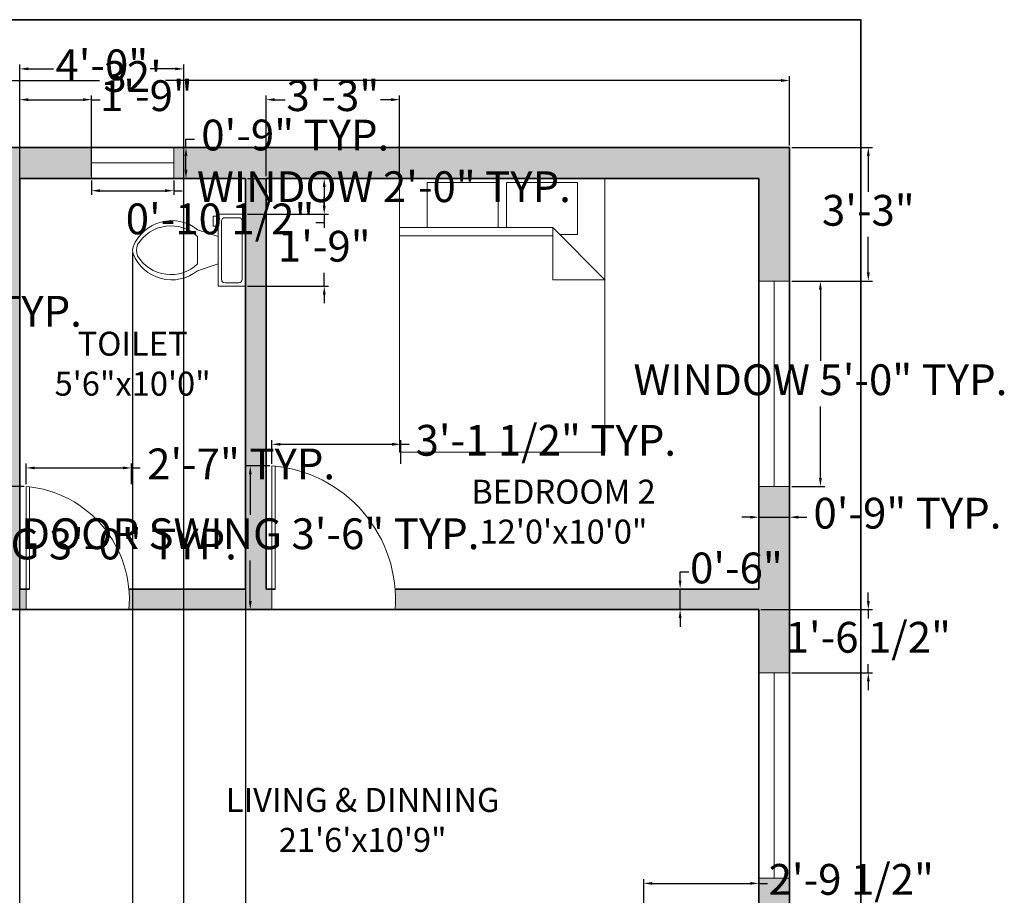
# Model space of a CAD drawing. Units: inches. Extents: x 1649 to 2193, y 1782 to 2280.
# Tile 3 of 3: x 1905 to 2193, y 2024 to 2280. Entities that reach past the tile are written whole.
import ezdxf

# ---------------------------------------------------------------- set-up
doc = ezdxf.new("R2010")
doc.units = ezdxf.units.IN
for name, color, linetype, lineweight in [('A-ANNO-DIMS', 2, 'Continuous', 18), ('A-ANNO-TTLB', 7, 'Continuous', 35), ('A-AREA-IDEN', 7, 'Continuous', 25), ('A-DOOR', 3, 'Continuous', 18), ('A-FLOR-FIXT', 9, 'Continuous', 18), ('A-FURN', 8, 'Continuous', 18), ('A-GLAZ', 4, 'Continuous', 18), ('A-WALL', 7, 'Continuous', 35)]:
    doc.layers.add(name, color=color, linetype=linetype, lineweight=lineweight)
doc.layers.add('A-WALL-PATT', color=18, linetype='Continuous', lineweight=13, true_color=0x000000)
doc.styles.get("Standard").update_dxf_attribs({"font": 'arial.ttf'})
doc.dimstyles.new('ISO-25', dxfattribs={"dimtxt": 9, "dimasz": 2.5, "dimexe": 1.25, "dimexo": 0.625, "dimgap": 2, "dimtad": 0, "dimtih": 1, "dimtoh": 1, "dimdec": 1, "dimlunit": 4, "dimtxsty": 'Standard', "dimcen": 2.5, "dimadec": 0, "dimazin": 0, "dimtfac": 0.5, "dimtdec": 1, "dimtmove": 0, "dimatfit": 3, "dimfxl": 1, "dimarcsym": 0})

# ---------------------------------------------------------------- blocks, each defined once
blk = doc.blocks.new('Bed - Queen')
for p, q in [((0, -80.00003), (0, 0)), ((0, 0), (59.99999, 0)), ((59.99999, 0), (59.99999, -80.00003)), ((7.99999, -1.2), (28.79998, -1.2)), ((7.99999, -14.4), (7.99999, -1.2)), ((28.79998, -1.2), (28.79998, -14.4)), ((31.19999, -1.2), (51.99999, -1.2)), ((31.19999, -14.4), (31.19999, -1.2)), ((51.99999, -1.2), (51.99999, -16.4)), ((0, -14.4), (44.8, -14.4)), ((44.8, -16.8), (0, -16.8)), ((59.99999, -29.6), (44.8, -14.4)), ((44.8, -14.4), (44.8, -29.6)), ((51.99999, -16.4), (46.79936, -16.4)), ((44.8, -29.6), (59.99999, -29.6)), ((59.99999, -80.00003), (0, -80.00003))]:
    blk.add_line(p, q)
blk = doc.blocks.new('*U6')
for p, q in [((9.5, -6), (9.5, -2)), ((-10, -8.5), (-8, -8.5)), ((-10, -9.5), (-10, -8.5)), ((-8, -8.5), (-8, -8)), ((-7, -8), (-7, -9.5)), ((-4, -8), (-6, -14)), ((4, -8), (6, -14)), ((-7, -9.5), (-10, -9.5)), ((4, -14), (-4, -14))]:
    blk.add_line(p, q)
blk.add_lwpolyline([(10.5, -8), (10.5, 0), (-10.5, 0), (-10.5, -8)], close=True)
for points in [[(-9.5, -2), (-9.5, -6)], [(8.5, -1), (-8.5, -1)], [(-8.5, -7), (8.5, -7)]]:
    blk.add_lwpolyline(points)
for centre, radius, start, end in [((-8.62, -1.88), 0.884, 81.8699, 188.1301), ((8.62, -1.88), 0.884, 351.8699, 98.1301), ((-8.62, -6.12), 0.884, 171.8699, 278.1301), ((8.62, -6.12), 0.884, 261.8699, 8.1301), ((3.52, -21.58), 12.17, 141.4691, 247.9714), ((4.2, -21.82), 11.33, 136.3677, 238.9468), ((-3.52, -21.58), 12.17, 292.0284, 38.5307), ((-4.2, -21.82), 11.33, 301.053, 43.6321), ((0, -27.88), 4, 245.7318, 294.2682), ((0, -29), 4, 254.8605, 285.1395)]:
    blk.add_arc(centre, radius, start, end)
blk = doc.blocks.new('*D7')
at = {"layer": 'A-ANNO-DIMS', "color": 0, "lineweight": -2, "transparency": 16777216}
for p, q in [((1746.13, 2243.28), (1746.13, 2263.5)), ((1748.63, 2262.25), (1928.49, 2262.25)), ((2127.63, 2262.25), (1947.76, 2262.25)), ((2130.13, 2243.28), (2130.13, 2263.5))]:
    blk.add_line(p, q, dxfattribs=at)
at = {"layer": 'A-ANNO-DIMS', "color": 0, "transparency": 16777216}
for points in [[(1748.63, 2262.67), (1748.63, 2261.83), (1746.13, 2262.25)], [(2127.63, 2262.67), (2127.63, 2261.83), (2130.13, 2262.25)]]:
    blk.add_solid(points, dxfattribs=at)
at = {"layer": 'Defpoints', "color": 0, "transparency": 16777216}
for p in [(2130.13, 2262.25), (1746.13, 2242.65), (2130.13, 2242.65)]:
    blk.add_point(p, dxfattribs=at)
at = {"layer": 'A-ANNO-DIMS', "color": 0, "transparency": 16777216, "insert": (1938.13, 2262.25), "char_height": 9, "attachment_point": 5}
blk.add_mtext("32'", dxfattribs=at)
blk = doc.blocks.new('DOOR-36IN')
for p, q in [((0, 6), (0, 42)), ((1, 6), (1, 42)), ((0, 6), (0, 0))]:
    blk.add_line(p, q)
blk.add_arc((-3, 3), 39.12, 355.6013, 85.6013)
blk = doc.blocks.new('WIN-60IN')
for p, q in [((0, 60), (9, 60)), ((4.5, 60), (4.5, 0)), ((0, 0), (9, 0))]:
    blk.add_line(p, q)
blk = doc.blocks.new('DOOR-30IN')
for p, q in [((0, 6), (0, 36)), ((1, 6), (1, 36)), ((0, 6), (0, 0))]:
    blk.add_line(p, q)
blk.add_arc((-3, 3), 33.14, 354.8056, 84.8056)
blk = doc.blocks.new('WIN-24IN')
for p, q in [((0, 0), (0, 9)), ((24, 0), (24, 9)), ((0, 4.5), (24, 4.5))]:
    blk.add_line(p, q)
blk = doc.blocks.new('*D15')
at = {"layer": 'A-ANNO-DIMS', "color": 0, "lineweight": -2, "transparency": 16777216}
for p, q in [((1978.19, 2149.65), (1971.26, 2149.65)), ((1972.51, 2147.15), (1972.51, 2135.31)), ((1972.51, 2110.15), (1972.51, 2121.99)), ((1978.19, 2107.65), (1971.26, 2107.65))]:
    blk.add_line(p, q, dxfattribs=at)
at = {"layer": 'A-ANNO-DIMS', "color": 0, "transparency": 16777216}
for points in [[(1972.1, 2147.15), (1972.93, 2147.15), (1972.51, 2149.65)], [(1972.1, 2110.15), (1972.93, 2110.15), (1972.51, 2107.65)]]:
    blk.add_solid(points, dxfattribs=at)
at = {"layer": 'Defpoints', "color": 0, "transparency": 16777216}
for p in [(1972.51, 2149.65), (1978.81, 2149.65), (1978.81, 2107.65)]:
    blk.add_point(p, dxfattribs=at)
at = {"layer": 'A-ANNO-DIMS', "color": 0, "transparency": 16777216, "insert": (1972.51, 2128.65), "char_height": 9, "attachment_point": 5}
blk.add_mtext('DOOR SWING 3\'-6" TYP.', dxfattribs=at)
blk = doc.blocks.new('*D16')
at = {"layer": 'A-ANNO-DIMS', "color": 0, "lineweight": -2, "transparency": 16777216}
for p, q in [((1978.81, 2150.28), (1978.81, 2157.2)), ((1981.31, 2155.95), (2013.97, 2155.95)), ((2016.47, 2150.28), (2016.47, 2157.2)), ((2016.47, 2155.95), (2018.97, 2155.95))]:
    blk.add_line(p, q, dxfattribs=at)
at = {"layer": 'A-ANNO-DIMS', "color": 0, "transparency": 16777216}
for points in [[(1981.31, 2156.37), (1981.31, 2155.54), (1978.81, 2155.95)], [(2013.97, 2156.37), (2013.97, 2155.54), (2016.47, 2155.95)]]:
    blk.add_solid(points, dxfattribs=at)
at = {"layer": 'Defpoints', "color": 0, "transparency": 16777216}
for p in [(2016.47, 2155.95), (1978.81, 2149.65), (2016.47, 2149.65)]:
    blk.add_point(p, dxfattribs=at)
at = {"layer": 'A-ANNO-DIMS', "color": 0, "transparency": 16777216, "insert": (2058.88, 2155.95), "char_height": 9, "attachment_point": 5}
blk.add_mtext('3\'-1 1/2" TYP.', dxfattribs=at)
blk = doc.blocks.new('*D17')
at = {"layer": 'A-ANNO-DIMS', "color": 0, "lineweight": -2, "transparency": 16777216}
for p, q in [((1906.4, 2143.65), (1900.38, 2143.65)), ((1901.63, 2141.15), (1901.63, 2132.31)), ((1901.63, 2110.15), (1901.63, 2118.99)), ((1906.4, 2107.65), (1900.38, 2107.65))]:
    blk.add_line(p, q, dxfattribs=at)
at = {"layer": 'A-ANNO-DIMS', "color": 0, "transparency": 16777216}
for points in [[(1901.21, 2141.15), (1902.05, 2141.15), (1901.63, 2143.65)], [(1901.21, 2110.15), (1902.05, 2110.15), (1901.63, 2107.65)]]:
    blk.add_solid(points, dxfattribs=at)
at = {"layer": 'Defpoints', "color": 0, "transparency": 16777216}
for p in [(1901.63, 2143.65), (1907.03, 2143.65), (1907.03, 2107.65)]:
    blk.add_point(p, dxfattribs=at)
at = {"layer": 'A-ANNO-DIMS', "color": 0, "transparency": 16777216, "insert": (1901.63, 2125.65), "char_height": 9, "attachment_point": 5}
blk.add_mtext('DOOR SWING 3\'-0" TYP.', dxfattribs=at)
blk = doc.blocks.new('*D18')
at = {"layer": 'A-ANNO-DIMS', "color": 0, "lineweight": -2, "transparency": 16777216}
for p, q in [((1907.03, 2144.28), (1907.03, 2150.3)), ((1937.82, 2144.28), (1937.82, 2150.3)), ((1909.53, 2149.05), (1935.32, 2149.05)), ((1937.82, 2149.05), (1940.32, 2149.05))]:
    blk.add_line(p, q, dxfattribs=at)
at = {"layer": 'A-ANNO-DIMS', "color": 0, "transparency": 16777216}
for points in [[(1909.53, 2149.47), (1909.53, 2148.64), (1907.03, 2149.05)], [(1935.32, 2149.47), (1935.32, 2148.64), (1937.82, 2149.05)]]:
    blk.add_solid(points, dxfattribs=at)
at = {"layer": 'Defpoints', "color": 0, "transparency": 16777216}
for p in [(1937.82, 2149.05), (1907.03, 2143.65), (1937.82, 2143.65)]:
    blk.add_point(p, dxfattribs=at)
at = {"layer": 'A-ANNO-DIMS', "color": 0, "transparency": 16777216, "insert": (1969.83, 2149.05), "char_height": 9, "attachment_point": 5}
blk.add_mtext('2\'-7" TYP.', dxfattribs=at)
blk = doc.blocks.new('*D19')
at = {"layer": 'A-ANNO-DIMS', "color": 0, "lineweight": -2, "transparency": 16777216}
for p, q in [((1926.13, 2233.03), (1926.13, 2228.8)), ((1950.13, 2233.03), (1950.13, 2228.8)), ((1928.63, 2230.05), (1947.63, 2230.05)), ((1950.13, 2230.05), (1952.63, 2230.05))]:
    blk.add_line(p, q, dxfattribs=at)
at = {"layer": 'A-ANNO-DIMS', "color": 0, "transparency": 16777216}
for points in [[(1928.63, 2230.47), (1928.63, 2229.64), (1926.13, 2230.05)], [(1947.63, 2230.47), (1947.63, 2229.64), (1950.13, 2230.05)]]:
    blk.add_solid(points, dxfattribs=at)
at = {"layer": 'Defpoints', "color": 0, "transparency": 16777216}
for p in [(1926.13, 2233.65), (1950.13, 2233.65), (1950.13, 2230.05)]:
    blk.add_point(p, dxfattribs=at)
at = {"layer": 'A-ANNO-DIMS', "color": 0, "transparency": 16777216, "insert": (2011.57, 2230.05), "char_height": 9, "attachment_point": 5}
blk.add_mtext('WINDOW 2\'-0" TYP.', dxfattribs=at)
blk = doc.blocks.new('*D20')
at = {"layer": 'A-ANNO-DIMS', "color": 0, "lineweight": -2, "transparency": 16777216}
for p, q in [((1953.73, 2242.65), (1953.73, 2245.15)), ((1953.73, 2245.15), (1956.23, 2245.15)), ((1950.75, 2242.65), (1954.98, 2242.65)), ((1953.73, 2236.15), (1953.73, 2240.15)), ((1950.75, 2233.65), (1954.98, 2233.65))]:
    blk.add_line(p, q, dxfattribs=at)
at = {"layer": 'A-ANNO-DIMS', "color": 0, "transparency": 16777216}
for points in [[(1953.31, 2240.15), (1954.15, 2240.15), (1953.73, 2242.65)], [(1953.31, 2236.15), (1954.15, 2236.15), (1953.73, 2233.65)]]:
    blk.add_solid(points, dxfattribs=at)
at = {"layer": 'Defpoints', "color": 0, "transparency": 16777216}
for p in [(1950.13, 2242.65), (1953.73, 2242.65), (1950.13, 2233.65)]:
    blk.add_point(p, dxfattribs=at)
at = {"layer": 'A-ANNO-DIMS', "color": 0, "transparency": 16777216, "insert": (1985.66, 2245.15), "char_height": 9, "attachment_point": 5}
blk.add_mtext('0\'-9" TYP.', dxfattribs=at)
blk = doc.blocks.new('*D25')
at = {"layer": 'A-ANNO-DIMS', "color": 0, "lineweight": -2, "transparency": 16777216}
for p, q in [((2130.75, 2203.65), (2140.38, 2203.65)), ((2139.13, 2201.15), (2139.13, 2180.31)), ((2139.13, 2146.15), (2139.13, 2167)), ((2130.75, 2143.65), (2140.38, 2143.65))]:
    blk.add_line(p, q, dxfattribs=at)
at = {"layer": 'A-ANNO-DIMS', "color": 0, "transparency": 16777216}
for points in [[(2138.71, 2201.15), (2139.55, 2201.15), (2139.13, 2203.65)], [(2138.71, 2146.15), (2139.55, 2146.15), (2139.13, 2143.65)]]:
    blk.add_solid(points, dxfattribs=at)
at = {"layer": 'Defpoints', "color": 0, "transparency": 16777216}
for p in [(2130.13, 2203.65), (2139.13, 2203.65), (2130.13, 2143.65)]:
    blk.add_point(p, dxfattribs=at)
at = {"layer": 'A-ANNO-DIMS', "color": 0, "transparency": 16777216, "insert": (2139.13, 2173.65), "char_height": 9, "attachment_point": 5}
blk.add_mtext('WINDOW 5\'-0" TYP.', dxfattribs=at)
blk = doc.blocks.new('*D26')
at = {"layer": 'A-ANNO-DIMS', "color": 0, "lineweight": -2, "transparency": 16777216}
for p, q in [((2121.13, 2143.03), (2121.13, 2133.4)), ((2130.13, 2143.03), (2130.13, 2133.4)), ((2118.63, 2134.65), (2116.13, 2134.65)), ((2121.13, 2134.65), (2130.13, 2134.65)), ((2132.63, 2134.65), (2135.13, 2134.65))]:
    blk.add_line(p, q, dxfattribs=at)
at = {"layer": 'A-ANNO-DIMS', "color": 0, "transparency": 16777216}
for points in [[(2118.63, 2135.07), (2118.63, 2134.24), (2121.13, 2134.65)], [(2132.63, 2135.07), (2132.63, 2134.24), (2130.13, 2134.65)]]:
    blk.add_solid(points, dxfattribs=at)
at = {"layer": 'Defpoints', "color": 0, "transparency": 16777216}
for p in [(2121.13, 2143.65), (2130.13, 2143.65), (2130.13, 2134.65)]:
    blk.add_point(p, dxfattribs=at)
at = {"layer": 'A-ANNO-DIMS', "color": 0, "transparency": 16777216, "insert": (2164.56, 2134.65), "char_height": 9, "attachment_point": 5}
blk.add_mtext('0\'-9" TYP.', dxfattribs=at)
blk = doc.blocks.new('*D27')
at = {"layer": 'A-ANNO-DIMS', "color": 0, "lineweight": -2, "transparency": 16777216}
for p, q in [((1849.19, 2233.65), (1861.81, 2233.65)), ((1860.56, 2231.15), (1860.56, 2200.58)), ((1860.56, 2156.15), (1860.56, 2186.72)), ((1849.19, 2153.65), (1861.81, 2153.65))]:
    blk.add_line(p, q, dxfattribs=at)
at = {"layer": 'A-ANNO-DIMS', "color": 0, "transparency": 16777216}
for points in [[(1860.14, 2231.15), (1860.98, 2231.15), (1860.56, 2233.65)], [(1860.14, 2156.15), (1860.98, 2156.15), (1860.56, 2153.65)]]:
    blk.add_solid(points, dxfattribs=at)
at = {"layer": 'Defpoints', "color": 0, "transparency": 16777216}
for p in [(1848.56, 2233.65), (1860.56, 2233.65), (1848.56, 2153.65)]:
    blk.add_point(p, dxfattribs=at)
at = {"layer": 'A-ANNO-DIMS', "color": 0, "transparency": 16777216, "insert": (1860.56, 2193.65), "char_height": 9, "attachment_point": 5}
blk.add_mtext('QUEEN BED 6\'-8" TYP.', dxfattribs=at)
blk = doc.blocks.new('*D36')
at = {"layer": 'A-ANNO-DIMS', "color": 0, "lineweight": -2, "transparency": 16777216}
for p, q in [((1905.13, 1979.28), (1905.13, 2266.9)), ((1907.63, 2265.65), (1914.99, 2265.65)), ((1950.63, 2265.65), (1943.27, 2265.65)), ((1953.13, 1979.28), (1953.13, 2266.9))]:
    blk.add_line(p, q, dxfattribs=at)
at = {"layer": 'A-ANNO-DIMS', "color": 0, "transparency": 16777216}
for points in [[(1907.63, 2266.07), (1907.63, 2265.24), (1905.13, 2265.65)], [(1950.63, 2266.07), (1950.63, 2265.24), (1953.13, 2265.65)]]:
    blk.add_solid(points, dxfattribs=at)
at = {"layer": 'Defpoints', "color": 0, "transparency": 16777216}
for p in [(1953.13, 2265.65), (1905.13, 1978.65), (1953.13, 1978.65)]:
    blk.add_point(p, dxfattribs=at)
at = {"layer": 'A-ANNO-DIMS', "color": 0, "transparency": 16777216, "insert": (1929.13, 2265.65), "char_height": 9, "attachment_point": 5}
blk.add_mtext('4\'-0"', dxfattribs=at)
blk = doc.blocks.new('*D37')
at = {"layer": 'A-ANNO-DIMS', "color": 0, "lineweight": -2, "transparency": 16777216}
for p, q in [((2098.13, 2116.15), (2098.13, 2118.65)), ((2098.13, 2118.65), (2100.63, 2118.65)), ((2120.5, 2113.65), (2096.88, 2113.65)), ((2098.13, 2107.65), (2098.13, 2113.65)), ((2120.5, 2107.65), (2096.88, 2107.65)), ((2098.13, 2105.15), (2098.13, 2102.65))]:
    blk.add_line(p, q, dxfattribs=at)
at = {"layer": 'A-ANNO-DIMS', "color": 0, "transparency": 16777216}
for points in [[(2097.71, 2116.15), (2098.55, 2116.15), (2098.13, 2113.65)], [(2097.71, 2105.15), (2098.55, 2105.15), (2098.13, 2107.65)]]:
    blk.add_solid(points, dxfattribs=at)
at = {"layer": 'Defpoints', "color": 0, "transparency": 16777216}
for p in [(2098.13, 2113.65), (2121.13, 2113.65), (2121.13, 2107.65)]:
    blk.add_point(p, dxfattribs=at)
at = {"layer": 'A-ANNO-DIMS', "color": 0, "transparency": 16777216, "insert": (2114.59, 2118.65), "char_height": 9, "attachment_point": 5}
blk.add_mtext('0\'-6"', dxfattribs=at)
blk = doc.blocks.new('*D43')
at = {"layer": 'A-ANNO-DIMS', "color": 0, "lineweight": -2, "transparency": 16777216}
for p, q in [((2153.13, 2110.15), (2153.13, 2112.65)), ((2121.75, 2107.65), (2154.38, 2107.65)), ((2153.13, 2107.65), (2153.13, 2105.06)), ((2130.75, 2089.15), (2154.38, 2089.15)), ((2153.13, 2089.15), (2153.13, 2091.75)), ((2153.13, 2086.65), (2153.13, 2084.15))]:
    blk.add_line(p, q, dxfattribs=at)
at = {"layer": 'A-ANNO-DIMS', "color": 0, "transparency": 16777216}
for points in [[(2152.71, 2110.15), (2153.55, 2110.15), (2153.13, 2107.65)], [(2152.71, 2086.65), (2153.55, 2086.65), (2153.13, 2089.15)]]:
    blk.add_solid(points, dxfattribs=at)
at = {"layer": 'Defpoints', "color": 0, "transparency": 16777216}
for p in [(2121.13, 2107.65), (2153.13, 2107.65), (2130.13, 2089.15)]:
    blk.add_point(p, dxfattribs=at)
at = {"layer": 'A-ANNO-DIMS', "color": 0, "transparency": 16777216, "insert": (2153.13, 2098.4), "char_height": 9, "attachment_point": 5}
blk.add_mtext('1\'-6 1/2"', dxfattribs=at)
blk = doc.blocks.new('*D44')
at = {"layer": 'A-ANNO-DIMS', "color": 0, "lineweight": -2, "transparency": 16777216}
for p, q in [((2130.75, 2242.65), (2154.38, 2242.65)), ((2153.13, 2240.15), (2153.13, 2229.75)), ((2153.13, 2206.15), (2153.13, 2216.55)), ((2130.75, 2203.65), (2154.38, 2203.65))]:
    blk.add_line(p, q, dxfattribs=at)
at = {"layer": 'A-ANNO-DIMS', "color": 0, "transparency": 16777216}
for points in [[(2152.71, 2240.15), (2153.55, 2240.15), (2153.13, 2242.65)], [(2152.71, 2206.15), (2153.55, 2206.15), (2153.13, 2203.65)]]:
    blk.add_solid(points, dxfattribs=at)
at = {"layer": 'Defpoints', "color": 0, "transparency": 16777216}
for p in [(2130.13, 2242.65), (2153.13, 2242.65), (2130.13, 2203.65)]:
    blk.add_point(p, dxfattribs=at)
at = {"layer": 'A-ANNO-DIMS', "color": 0, "transparency": 16777216, "insert": (2153.13, 2223.15), "char_height": 9, "attachment_point": 5}
blk.add_mtext('3\'-3"', dxfattribs=at)
blk = doc.blocks.new('*D49')
at = {"layer": 'A-ANNO-DIMS', "color": 0, "lineweight": -2, "transparency": 16777216}
for p, q in [((1905.13, 2234.28), (1905.13, 2257.9)), ((1907.63, 2256.65), (1923.63, 2256.65)), ((1926.13, 2234.28), (1926.13, 2257.9)), ((1926.13, 2256.65), (1928.63, 2256.65))]:
    blk.add_line(p, q, dxfattribs=at)
at = {"layer": 'A-ANNO-DIMS', "color": 0, "transparency": 16777216}
for points in [[(1907.63, 2257.07), (1907.63, 2256.24), (1905.13, 2256.65)], [(1923.63, 2257.07), (1923.63, 2256.24), (1926.13, 2256.65)]]:
    blk.add_solid(points, dxfattribs=at)
at = {"layer": 'Defpoints', "color": 0, "transparency": 16777216}
for p in [(1926.13, 2256.65), (1905.13, 2233.65), (1926.13, 2233.65)]:
    blk.add_point(p, dxfattribs=at)
at = {"layer": 'A-ANNO-DIMS', "color": 0, "transparency": 16777216, "insert": (1942.17, 2256.65), "char_height": 9, "attachment_point": 5}
blk.add_mtext('1\'-9"', dxfattribs=at)
blk = doc.blocks.new('*D50')
at = {"layer": 'A-ANNO-DIMS', "color": 0, "lineweight": -2, "transparency": 16777216}
for p, q in [((1994.13, 2225.65), (1994.13, 2228.15)), ((1971.75, 2223.15), (1995.38, 2223.15)), ((1994.13, 2223.15), (1994.13, 2219.24)), ((1994.13, 2202.15), (1994.13, 2206.05)), ((1971.75, 2202.15), (1995.38, 2202.15)), ((1994.13, 2199.65), (1994.13, 2197.15))]:
    blk.add_line(p, q, dxfattribs=at)
at = {"layer": 'A-ANNO-DIMS', "color": 0, "transparency": 16777216}
for points in [[(1993.71, 2225.65), (1994.55, 2225.65), (1994.13, 2223.15)], [(1993.71, 2199.65), (1994.55, 2199.65), (1994.13, 2202.15)]]:
    blk.add_solid(points, dxfattribs=at)
at = {"layer": 'Defpoints', "color": 0, "transparency": 16777216}
for p in [(1971.13, 2223.15), (1971.13, 2202.15), (1994.13, 2202.15)]:
    blk.add_point(p, dxfattribs=at)
at = {"layer": 'A-ANNO-DIMS', "color": 0, "transparency": 16777216, "insert": (1994.13, 2212.65), "char_height": 9, "attachment_point": 5}
blk.add_mtext('1\'-9"', dxfattribs=at)
blk = doc.blocks.new('*D51')
at = {"layer": 'A-ANNO-DIMS', "color": 0, "lineweight": -2, "transparency": 16777216}
for p, q in [((1938.13, 2212.02), (1938.13, 1786.4)), ((1971.13, 2201.52), (1971.13, 1786.4)), ((1935.63, 1787.65), (1933.13, 1787.65)), ((1938.13, 1787.65), (1940.59, 1787.65)), ((1971.13, 1787.65), (1968.67, 1787.65)), ((1973.63, 1787.65), (1976.13, 1787.65))]:
    blk.add_line(p, q, dxfattribs=at)
at = {"layer": 'A-ANNO-DIMS', "color": 0, "transparency": 16777216}
for points in [[(1935.63, 1788.07), (1935.63, 1787.24), (1938.13, 1787.65)], [(1973.63, 1788.07), (1973.63, 1787.24), (1971.13, 1787.65)]]:
    blk.add_solid(points, dxfattribs=at)
at = {"layer": 'Defpoints', "color": 0, "transparency": 16777216}
for p in [(1938.13, 2212.65), (1971.13, 2202.15), (1971.13, 1787.65)]:
    blk.add_point(p, dxfattribs=at)
at = {"layer": 'A-ANNO-DIMS', "color": 0, "transparency": 16777216, "insert": (1954.63, 1787.65), "char_height": 9, "attachment_point": 5}
blk.add_mtext('2\'-9"', dxfattribs=at)
blk = doc.blocks.new('*D53')
at = {"layer": 'A-ANNO-DIMS', "color": 0, "lineweight": -2, "transparency": 16777216}
for p, q in [((1977.13, 2234.28), (1977.13, 2257.9)), ((1979.63, 2256.65), (1982.68, 2256.65)), ((2013.66, 2256.65), (2010.6, 2256.65)), ((2016.16, 2234.28), (2016.16, 2257.9))]:
    blk.add_line(p, q, dxfattribs=at)
at = {"layer": 'A-ANNO-DIMS', "color": 0, "transparency": 16777216}
for points in [[(1979.63, 2257.07), (1979.63, 2256.24), (1977.13, 2256.65)], [(2013.66, 2257.07), (2013.66, 2256.24), (2016.16, 2256.65)]]:
    blk.add_solid(points, dxfattribs=at)
at = {"layer": 'Defpoints', "color": 0, "transparency": 16777216}
for p in [(2016.16, 2256.65), (1977.13, 2233.65), (2016.16, 2233.65)]:
    blk.add_point(p, dxfattribs=at)
at = {"layer": 'A-ANNO-DIMS', "color": 0, "transparency": 16777216, "insert": (1996.64, 2256.65), "char_height": 9, "attachment_point": 5}
blk.add_mtext('3\'-3"', dxfattribs=at)
blk = doc.blocks.new('*D54')
at = {"layer": 'A-ANNO-DIMS', "color": 0, "lineweight": -2, "transparency": 16777216}
for p, q in [((2087.48, 2005.28), (2087.48, 2028.9)), ((2121.13, 2005.28), (2121.13, 2028.9)), ((2089.98, 2027.65), (2118.63, 2027.65)), ((2121.13, 2027.65), (2123.63, 2027.65))]:
    blk.add_line(p, q, dxfattribs=at)
at = {"layer": 'A-ANNO-DIMS', "color": 0, "transparency": 16777216}
for points in [[(2089.98, 2028.07), (2089.98, 2027.24), (2087.48, 2027.65)], [(2118.63, 2028.07), (2118.63, 2027.24), (2121.13, 2027.65)]]:
    blk.add_solid(points, dxfattribs=at)
at = {"layer": 'Defpoints', "color": 0, "transparency": 16777216}
for p in [(2121.13, 2027.65), (2087.48, 2004.65), (2121.13, 2004.65)]:
    blk.add_point(p, dxfattribs=at)
at = {"layer": 'A-ANNO-DIMS', "color": 0, "transparency": 16777216, "insert": (2148.15, 2027.65), "char_height": 9, "attachment_point": 5}
blk.add_mtext('2\'-9 1/2"', dxfattribs=at)
blk = doc.blocks.new('*D60')
at = {"layer": 'A-ANNO-DIMS', "color": 0, "lineweight": -2, "transparency": 16777216}
for p, q in [((1971.75, 2233.65), (1995.38, 2233.65)), ((1994.13, 2231.15), (1994.13, 2225.65)), ((1971.75, 2223.15), (1995.38, 2223.15)), ((1994.13, 2223.15), (1994.13, 2220.65)), ((1994.13, 2220.65), (1991.63, 2220.65))]:
    blk.add_line(p, q, dxfattribs=at)
at = {"layer": 'A-ANNO-DIMS', "color": 0, "transparency": 16777216}
for points in [[(1993.71, 2231.15), (1994.55, 2231.15), (1994.13, 2233.65)], [(1993.71, 2225.65), (1994.55, 2225.65), (1994.13, 2223.15)]]:
    blk.add_solid(points, dxfattribs=at)
at = {"layer": 'Defpoints', "color": 0, "transparency": 16777216}
for p in [(1971.13, 2233.65), (1971.13, 2223.15), (1994.13, 2223.15)]:
    blk.add_point(p, dxfattribs=at)
at = {"layer": 'A-ANNO-DIMS', "color": 0, "transparency": 16777216, "insert": (1963.68, 2220.65), "char_height": 9, "attachment_point": 5}
blk.add_mtext('0\'-10 1/2"', dxfattribs=at)

msp = doc.modelspace()

# ---------------------------------------------------------------- hatches: boundary and pattern name
at = {"layer": 'A-WALL-PATT'}
h = msp.add_hatch(color=256, dxfattribs=at)
h.dxf.hatch_style = 1
h.paths.add_polyline_path([(1926.13, 2242.65), (1746.13, 2242.65), (1746.13, 2203.65), (1755.13, 2203.65), (1755.13, 2233.65), (1899.13, 2233.65), (1899.13, 2113.65), (1897.63, 2113.65), (1897.63, 2107.65), (1899.13, 2107.65), (1907.03, 2107.65), (1907.03, 2113.65), (1905.13, 2113.65), (1905.13, 2233.65), (1926.13, 2233.65)])
h.paths.add_polyline_path([(2130.13, 2242.65), (1950.13, 2242.65), (1950.13, 2233.65), (1971.13, 2233.65), (1971.13, 2113.65), (1937.03, 2113.65, -0.045361), (1937.03, 2107.65), (1978.81, 2107.65), (1978.81, 2113.65), (1977.13, 2113.65), (1977.13, 2233.65), (2121.13, 2233.65), (2121.13, 2203.65), (2130.13, 2203.65)])
h.paths.add_polyline_path([(2130.13, 2143.65), (2121.13, 2143.65), (2121.13, 2113.65), (2014.81, 2113.65, -0.038405), (2014.81, 2107.65), (2121.13, 2107.65), (2121.13, 2089.15), (2130.13, 2089.15)])
h.paths.add_polyline_path([(1824.23, 2113.65), (1755.13, 2113.65), (1755.13, 2143.65), (1746.13, 2143.65), (1746.13, 2093.65), (1755.13, 2093.65), (1755.13, 2107.65), (1824.23, 2107.65, -0.045361)])
h.paths.add_polyline_path([(1862.13, 2055.65), (1862.13, 2107.65), (1863.33, 2107.65, -0.038218), (1863.33, 2113.65), (1854.23, 2113.65), (1854.23, 2107.65), (1856.13, 2107.65), (1856.13, 2055.65), (1755.13, 2055.65), (1755.13, 2069.65), (1746.13, 2069.65), (1746.13, 2032.15), (1755.13, 2032.15), (1755.13, 2049.65), (1862.13, 2049.65)])
h.paths.add_polyline_path([(2130.13, 2029.15), (2121.13, 2029.15), (2121.13, 2010.65), (2087.48, 2010.65), (2087.48, 2004.65), (2121.13, 2004.65), (2121.13, 1968.65), (2087.48, 1968.65), (2087.48, 1962.65), (2121.13, 1962.65), (2121.13, 1942.65), (2130.13, 1942.65)])
h.paths.add_polyline_path([(2022.13, 1874.65), (1959.13, 1874.65), (1959.13, 1978.65), (1953.13, 1978.65), (1953.13, 1874.65), (1943.69, 1874.65, -0.055385), (1943.69, 1865.65), (2022.13, 1865.65)])
h.paths.add_polyline_path([(2130.13, 1894.65), (2121.13, 1894.65), (2121.13, 1874.65), (2058.13, 1874.65), (2058.13, 1865.65), (2121.13, 1865.65), (2130.13, 1865.65)])
h.paths.add_polyline_path([(1755.13, 1972.65), (1859.98, 1972.65, -0.038405), (1859.98, 1978.65), (1755.13, 1978.65), (1755.13, 1996.15), (1746.13, 1996.15), (1746.13, 1920.15), (1755.13, 1920.15)])
h.paths.add_polyline_path([(1803.13, 1819.65), (1755.13, 1819.65), (1755.13, 1872.15), (1746.13, 1872.15), (1746.13, 1810.65), (1803.13, 1810.65)])
h.paths.add_polyline_path([(1905.13, 1819.65), (1905.13, 1821.19), (1899.13, 1821.19), (1899.13, 1819.65), (1851.13, 1819.65), (1851.13, 1810.65), (1905.13, 1810.65)])
h.paths.add_polyline_path([(1907.69, 1874.65), (1905.13, 1874.65), (1905.13, 1972.65), (1905.13, 1978.65), (1895.98, 1978.65), (1895.98, 1972.65), (1899.13, 1972.65), (1899.13, 1857.19, -0.038405), (1905.13, 1857.19), (1905.13, 1865.65), (1907.69, 1865.65)])

# ---------------------------------------------------------------- linework, layer by layer
at = {"layer": 'A-ANNO-TTLB'}
msp.add_lwpolyline([(1708.93, 2280.02), (2150.99, 2280.02), (2150.99, 1796.25), (1708.93, 1796.25)], close=True, dxfattribs=at)
at = {"layer": 'A-WALL'}
for p, q in [((1746.13, 2242.65), (2130.13, 2242.65)), ((2130.13, 2242.65), (2130.13, 1810.65)), ((1905.13, 2113.65), (1905.13, 2233.65)), ((1905.13, 2233.65), (1971.13, 2233.65)), ((1971.13, 2113.65), (1971.13, 2233.65)), ((1977.13, 2113.65), (1977.13, 2233.65)), ((1977.13, 2233.65), (2121.13, 2233.65)), ((2121.13, 2233.65), (2121.13, 2113.65)), ((1905.13, 2113.65), (1908.03, 2113.65)), ((1937.03, 2113.65), (1971.13, 2113.65)), ((1977.13, 2113.65), (1979.81, 2113.65)), ((2014.81, 2113.65), (2121.13, 2113.65)), ((1899.13, 2107.65), (2121.13, 2107.65)), ((2121.13, 2107.65), (2121.13, 2010.65))]:
    msp.add_line(p, q, dxfattribs=at)

# ---------------------------------------------------------------- block references
at = {"layer": 'A-DOOR'}
for name, p in [('DOOR-36IN', (1978.81, 2107.65)), ('DOOR-30IN', (1907.03, 2107.65))]:
    msp.add_blockref(name, p, dxfattribs=at)
at = {"layer": 'A-FLOR-FIXT', "rotation": 270}
msp.add_blockref('*U6', (1971.13, 2212.65), dxfattribs=at)
at = {"layer": 'A-FURN'}
msp.add_blockref('Bed - Queen', (2016.16, 2233.65), dxfattribs=at)
at = {"layer": 'A-GLAZ'}
for name, p in [('WIN-24IN', (1926.13, 2233.65)), ('WIN-60IN', (2121.13, 2143.65))]:
    msp.add_blockref(name, p, dxfattribs=at)
at = {"layer": 'A-GLAZ', "rotation": 180}
msp.add_blockref('WIN-60IN', (2130.13, 2089.15), dxfattribs=at)

# ---------------------------------------------------------------- texts
at = {"layer": 'A-AREA-IDEN', "char_height": 7, "attachment_point": 1}
for s, width, insert in [('\\pxqc;{\\fArial|b1|i0|c0|p34;TOILET\\P5\'6"x10\'0"}', 66, (1905.13, 2188.83)), ('\\pxqc;{\\fArial|b1|i0|c0|p34;BEDROOM 2\\P12\'0\'x10\'0"}', 91.4848, (2018.3, 2145.61)), ('\\pxqc;{\\fArial|b1|i0|c0|p34;LIVING & DINNING\\P21\'6\'x10\'9"}', 96.7712, (1956.97, 2055.53))]:
    msp.add_mtext_dynamic_manual_height_columns(s, width=width, gutter_width=12.5, heights=[0], dxfattribs=dict(at, insert=insert))

# ---------------------------------------------------------------- dimensions: what is measured, and where the dimension line sits
at = {"layer": 'A-ANNO-DIMS'}
for base, p1, p2, override, picture, middle in [((1953.13, 2265.65), (1905.13, 1978.65), (1953.13, 1978.65), {"dimdec": 1, "dimlfac": 1, "dimrnd": 0, "dimzin": 1, "dimdsep": 46, "dimlunit": 4, "dimfrac": 2}, '*D36', (1929.13, 2265.65)), ((2130.13, 2262.25), (1746.13, 2242.65), (2130.13, 2242.65), {"dimclrd": 0, "dimclre": 0, "dimclrt": 0}, '*D7', (1938.13, 2262.25)), ((1926.13, 2256.65), (1905.13, 2233.65), (1926.13, 2233.65), {"dimdec": 1, "dimlfac": 1, "dimrnd": 0, "dimzin": 1, "dimdsep": 46, "dimlunit": 4, "dimfrac": 2}, '*D49', (1942.17, 2256.65)), ((1971.13, 1787.65), (1938.13, 2212.65), (1971.13, 2202.15), {"dimdec": 1, "dimlfac": 1, "dimrnd": 0, "dimzin": 1, "dimdsep": 46, "dimlunit": 4, "dimfrac": 2}, '*D51', (1954.63, 1787.65)), ((2121.1289, 2027.6524), (2087.4781, 2004.6524), (2121.1289, 2004.6524), {"dimdec": 1, "dimlfac": 1, "dimrnd": 0, "dimzin": 1, "dimdsep": 46, "dimlunit": 4, "dimfrac": 2}, '*D54', (2148.1535, 2027.6524))]:
    dim = msp.add_linear_dim(base=base, p1=p1, p2=p2, dimstyle='ISO-25', override=override, dxfattribs=at)
    dim.commit()
    dim.dimension.update_dxf_attribs({"geometry": picture, "text_midpoint": middle})
for base, p1, p2, angle, picture, middle in [((2016.16, 2256.65), (1977.13, 2233.65), (2016.16, 2233.65), 0, '*D53', (1996.64, 2256.65)), ((2153.13, 2242.65), (2130.13, 2203.65), (2130.13, 2242.65), 90, '*D44', (2153.13, 2223.15)), ((1994.13, 2223.15), (1971.13, 2233.65), (1971.13, 2223.15), 270, '*D60', (1963.68, 2220.65)), ((1994.13, 2202.15), (1971.13, 2223.15), (1971.13, 2202.15), 270, '*D50', (1994.13, 2212.65)), ((2098.13, 2113.65), (2121.13, 2107.65), (2121.13, 2113.65), 90, '*D37', (2114.59, 2118.65)), ((2153.13, 2107.65), (2130.13, 2089.15), (2121.13, 2107.65), 90, '*D43', (2153.13, 2098.4))]:
    dim = msp.add_linear_dim(base=base, p1=p1, p2=p2, angle=angle, dimstyle='ISO-25', override={"dimdec": 1, "dimlfac": 1, "dimrnd": 0, "dimzin": 1, "dimdsep": 46, "dimlunit": 4, "dimfrac": 2}, dxfattribs=at)
    dim.commit()
    dim.dimension.update_dxf_attribs({"geometry": picture, "text_midpoint": middle})
for base, p1, p2, text, picture, middle in [((1953.73, 2242.65), (1950.13, 2233.65), (1950.13, 2242.65), '<> TYP.', '*D20', (1985.66, 2245.15)), ((1860.56, 2233.65), (1848.56, 2153.65), (1848.56, 2233.65), 'QUEEN BED <> TYP.', '*D27', (1860.56, 2193.65)), ((2139.13, 2203.65), (2130.13, 2143.65), (2130.13, 2203.65), 'WINDOW <> TYP.', '*D25', (2139.13, 2173.65)), ((1972.51, 2149.65), (1978.81, 2107.65), (1978.81, 2149.65), 'DOOR SWING <> TYP.', '*D15', (1972.51, 2128.65)), ((1901.63, 2143.65), (1907.03, 2107.65), (1907.03, 2143.65), 'DOOR SWING <> TYP.', '*D17', (1901.63, 2125.65))]:
    dim = msp.add_linear_dim(base=base, p1=p1, p2=p2, angle=90, text=text, dimstyle='ISO-25', override={"dimdec": 1, "dimlfac": 1, "dimrnd": 0, "dimzin": 1, "dimdsep": 46, "dimlunit": 4, "dimfrac": 2}, dxfattribs=at)
    dim.commit()
    dim.dimension.update_dxf_attribs({"geometry": picture, "text_midpoint": middle})
for base, p1, p2, text, picture, middle in [((1950.13, 2230.05), (1926.13, 2233.65), (1950.13, 2233.65), 'WINDOW <> TYP.', '*D19', (2011.57, 2230.05)), ((2016.47, 2155.95), (1978.81, 2149.65), (2016.47, 2149.65), '<> TYP.', '*D16', (2058.88, 2155.95)), ((1937.82, 2149.05), (1907.03, 2143.65), (1937.82, 2143.65), '<> TYP.', '*D18', (1969.83, 2149.05)), ((2130.13, 2134.65), (2121.13, 2143.65), (2130.13, 2143.65), '<> TYP.', '*D26', (2164.56, 2134.65))]:
    dim = msp.add_linear_dim(base=base, p1=p1, p2=p2, text=text, dimstyle='ISO-25', override={"dimdec": 1, "dimlfac": 1, "dimrnd": 0, "dimzin": 1, "dimdsep": 46, "dimlunit": 4, "dimfrac": 2}, dxfattribs=at)
    dim.commit()
    dim.dimension.update_dxf_attribs({"geometry": picture, "text_midpoint": middle})

doc.saveas('drawing.dxf')
